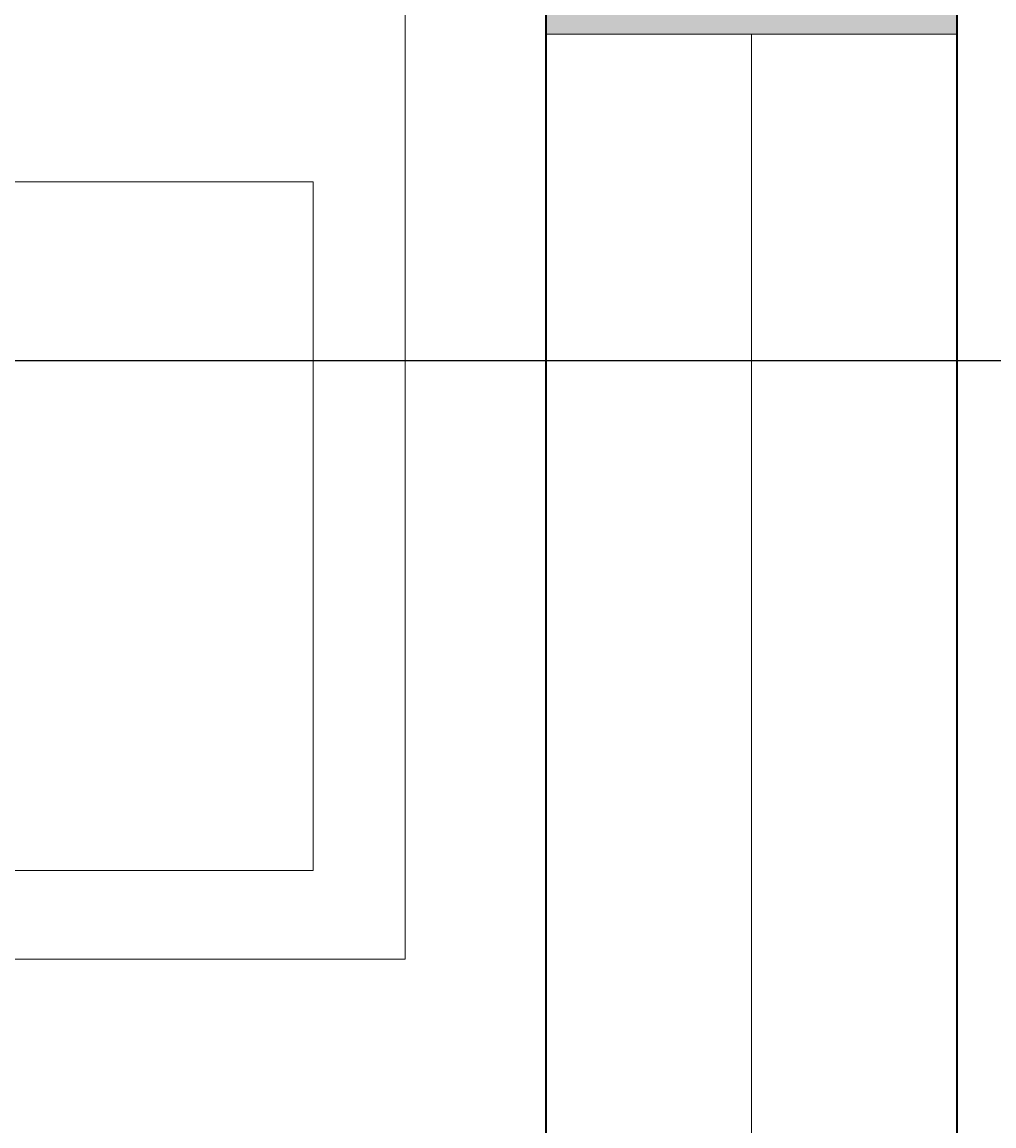
# Model space of a CAD drawing. Units: inches. Extents: x 1568 to 2529, y 2149 to 2897.
# Tile 11 of 16: x 1953 to 1974, y 2434 to 2459. Entities that reach past the tile are written whole.
import ezdxf

# ---------------------------------------------------------------- set-up
doc = ezdxf.new("R2010")
doc.units = ezdxf.units.IN
for name, color, linetype, lineweight in [('A-ANNO-DIMS', 2, 'Continuous', 18), ('A-FLOR-FIXT', 9, 'Continuous', 18), ('A-WALL-PATT', 172, 'Continuous', 13), ('wall', 7, 'Continuous', 35), ('window', 130, 'Continuous', 18)]:
    doc.layers.add(name, color=color, linetype=linetype, lineweight=lineweight)
doc.styles.get("Standard").update_dxf_attribs({"font": 'arial.ttf'})
doc.dimstyles.get("Standard").update_dxf_attribs({"dimtxt": 0.18, "dimasz": 0.18, "dimexe": 0.18, "dimexo": 0.0625, "dimgap": 0.09, "dimtad": 0, "dimtih": 1, "dimtoh": 1, "dimdec": 4, "dimzin": 0, "dimdsep": 46, "dimtxsty": 'Standard', "dimcen": 0.09, "dimadec": 0, "dimazin": 0, "dimtfac": 1, "dimtdec": 4, "dimtofl": 0, "dimtmove": 0, "dimatfit": 3, "dimfxl": 1, "dimtolj": 1, "dimtzin": 0, "dimarcsym": 0})

# ---------------------------------------------------------------- blocks, each defined once
blk = doc.blocks.new('*D28')
at = {"layer": 'A-ANNO-DIMS', "color": 0, "lineweight": -2, "transparency": 16777216}
for p, q in [((1973.643, 2801.532), (2009.61, 2801.532)), ((2009.43, 2801.352), (2009.43, 2501.714)), ((2009.43, 2201.712), (2009.43, 2501.35)), ((1973.613, 2201.532), (2009.61, 2201.532))]:
    blk.add_line(p, q, dxfattribs=at)
at = {"layer": 'A-ANNO-DIMS', "color": 0, "transparency": 16777216}
for points in [[(2009.4, 2801.352), (2009.46, 2801.352), (2009.43, 2801.532)], [(2009.4, 2201.712), (2009.46, 2201.712), (2009.43, 2201.532)]]:
    blk.add_solid(points, dxfattribs=at)
at = {"layer": 'Defpoints', "color": 0, "transparency": 16777216}
for p in [(1973.58, 2801.532), (2009.43, 2801.532), (1973.551, 2201.532)]:
    blk.add_point(p, dxfattribs=at)
at = {"layer": 'A-ANNO-DIMS', "color": 0, "transparency": 16777216, "insert": (2009.43, 2501.532), "char_height": 0.18, "attachment_point": 5}
blk.add_mtext('\\A1;600', dxfattribs=at)
blk = doc.blocks.new('*D32')
at = {"layer": 'A-ANNO-DIMS', "color": 0, "lineweight": -2, "transparency": 16777216}
for p, q in [((1964.551, 2792.469), (1964.551, 2165.502)), ((1904.551, 2753.401), (1904.551, 2165.502)), ((1904.731, 2165.682), (1934.332, 2165.682)), ((1964.371, 2165.682), (1934.77, 2165.682))]:
    blk.add_line(p, q, dxfattribs=at)
at = {"layer": 'A-ANNO-DIMS', "color": 0, "transparency": 16777216}
for points in [[(1904.731, 2165.712), (1904.731, 2165.652), (1904.551, 2165.682)], [(1964.371, 2165.712), (1964.371, 2165.652), (1964.551, 2165.682)]]:
    blk.add_solid(points, dxfattribs=at)
at = {"layer": 'Defpoints', "color": 0, "transparency": 16777216}
for p in [(1964.551, 2792.532), (1904.551, 2753.463), (1964.551, 2165.682)]:
    blk.add_point(p, dxfattribs=at)
at = {"layer": 'A-ANNO-DIMS', "color": 0, "transparency": 16777216, "insert": (1934.551, 2165.682), "char_height": 0.18, "attachment_point": 5}
blk.add_mtext('\\A1;60', dxfattribs=at)
blk = doc.blocks.new('*D35')
at = {"layer": 'A-ANNO-DIMS', "color": 0, "lineweight": -2, "transparency": 16777216}
for p, q in [((1759.113, 2451.227), (2009.61, 2451.227)), ((2009.43, 2451.047), (2009.43, 2431.409)), ((2009.43, 2411.407), (2009.43, 2431.045)), ((1759.113, 2411.227), (2009.61, 2411.227))]:
    blk.add_line(p, q, dxfattribs=at)
at = {"layer": 'A-ANNO-DIMS', "color": 0, "transparency": 16777216}
for points in [[(2009.4, 2451.047), (2009.46, 2451.047), (2009.43, 2451.227)], [(2009.4, 2411.407), (2009.46, 2411.407), (2009.43, 2411.227)]]:
    blk.add_solid(points, dxfattribs=at)
at = {"layer": 'Defpoints', "color": 0, "transparency": 16777216}
for p in [(1759.051, 2451.227), (2009.43, 2451.227), (1759.051, 2411.227)]:
    blk.add_point(p, dxfattribs=at)
at = {"layer": 'A-ANNO-DIMS', "color": 0, "transparency": 16777216, "insert": (2009.43, 2431.227), "char_height": 0.18, "attachment_point": 5}
blk.add_mtext('\\A1;40', dxfattribs=at)

msp = doc.modelspace()

# ---------------------------------------------------------------- hatches: boundary and pattern name
at = {"layer": 'A-WALL-PATT'}
h = msp.add_hatch(color=256, dxfattribs=at)
h.dxf.hatch_style = 1
h.paths.add_polyline_path([(1738.1593, 2801.532), (1634.4841, 2801.532), (1634.4841, 2792.532), (1738.1593, 2792.532)])
h.paths.add_polyline_path([(1812.4114, 2801.532), (1759.0925, 2801.532), (1759.0925, 2792.532), (1812.4114, 2792.532)])
h.paths.add_polyline_path([(1952.647, 2801.532), (1848.4114, 2801.532), (1848.4114, 2792.532), (1952.647, 2792.532)])
h.paths.add_polyline_path([(1973.5509, 2792.532), (1964.5509, 2792.532), (1964.5509, 2699.1671), (1973.5509, 2699.1671)])
h.paths.add_polyline_path([(1973.5509, 2663.1671), (1964.5509, 2663.1671), (1964.5509, 2630.5978), (1973.5509, 2630.5978)])
h.paths.add_polyline_path([(1973.5509, 2609.6646), (1964.5509, 2609.6646), (1964.5509, 2572.3679), (1973.5509, 2572.3679)])
h.paths.add_polyline_path([(1622.5509, 2753.3576), (1622.3864, 2753.3576), (1613.5509, 2753.3576), (1613.5509, 2705.9172), (1622.5509, 2705.9172)])
h.paths.add_polyline_path([(1622.5509, 2669.9172), (1613.5509, 2669.9172), (1613.5509, 2624.532), (1622.5509, 2624.532)])
h.paths.add_polyline_path([(1759.0509, 2757.9833), (1754.5509, 2757.9833), (1754.5509, 2744.532), (1622.5509, 2744.532), (1622.5509, 2740.032), (1754.5509, 2740.032), (1754.5509, 2730.8156), (1759.0509, 2730.8156), (1759.0509, 2740.032)])
h.paths.add_polyline_path([(1759.0509, 2690.8156), (1754.5509, 2690.8156), (1754.5509, 2624.532), (1759.0509, 2624.532)])
h.paths.add_polyline_path([(1738.1177, 2620.032), (1634.4841, 2620.032), (1634.4841, 2615.532), (1738.1177, 2615.532)])
h.paths.add_polyline_path([(1622.5509, 2615.532), (1613.5509, 2615.532), (1613.5509, 2564.2764), (1622.5509, 2564.2764)])
h.paths.add_polyline_path([(1759.0509, 2411.2271), (1754.5509, 2411.2271), (1754.5509, 2339.532), (1759.0509, 2339.532)])
h.paths.add_polyline_path([(1759.0509, 2464.032), (1734.3925, 2464.032), (1622.5509, 2464.032), (1622.5509, 2459.532), (1736.5509, 2459.532), (1754.5509, 2459.532), (1754.5509, 2451.2271), (1759.0509, 2451.2271)])
h.paths.add_polyline_path([(1844.5509, 2471.532), (1858.1805, 2471.532), (1858.1805, 2476.032), (1844.5509, 2476.032), (1844.5509, 2510.0763), (1840.0509, 2510.0763), (1840.0509, 2476.032), (1840.0509, 2339.532), (1844.5509, 2339.532)])
h.paths.add_polyline_path([(1844.5509, 2596.032), (1964.5509, 2596.032), (1964.5509, 2600.532), (1840.0509, 2600.532), (1840.0509, 2570.0763), (1844.5509, 2570.0763)])
h.paths.add_polyline_path([(1964.5509, 2476.032), (1894.1805, 2476.032), (1894.1805, 2471.532), (1964.5509, 2471.532)])
h.paths.add_polyline_path([(1622.5509, 2528.2764), (1613.5509, 2528.2764), (1613.5509, 2436.512), (1622.5509, 2436.512)])
h.paths.add_polyline_path([(1622.5509, 2400.512), (1613.5509, 2400.512), (1613.5509, 2339.532), (1622.5509, 2339.532)])
h.paths.add_polyline_path([(1738.9144, 2339.532), (1634.4841, 2339.532), (1634.4841, 2330.532), (1738.9144, 2330.532)])
h.paths.add_polyline_path([(1792.463, 2336.532, -0.0187698), (1792.5756, 2339.532), (1783.8928, 2339.532), (1783.8928, 2330.532), (1792.463, 2330.532)])
h.paths.add_polyline_path([(1952.6177, 2339.532), (1885.2912, 2339.532), (1885.2912, 2330.532), (1952.6177, 2330.532)])
h.paths.add_polyline_path([(1973.5509, 2422.371), (1964.5509, 2422.371), (1964.5509, 2395.032), (1964.5509, 2387.286), (1964.5509, 2339.532), (1973.5509, 2339.532)])
h.paths.add_polyline_path([(1973.5509, 2536.3679), (1964.5509, 2536.3679), (1964.5509, 2476.032), (1964.5509, 2458.371), (1973.5509, 2458.371)])

# ---------------------------------------------------------------- linework, layer by layer
at = {"layer": 'A-FLOR-FIXT'}
for points in [[(1941.7397, 2469.6671), (1961.4644, 2469.6671), (1961.4644, 2438.1142), (1941.7397, 2438.1142)], [(1943.5781, 2440.0573), (1959.4492, 2440.0573), (1959.4492, 2455.1398), (1943.5781, 2455.1398)]]:
    msp.add_lwpolyline(points, close=True, dxfattribs=at)
at = {"layer": 'wall'}
msp.add_lwpolyline([(1613.5509, 2201.532), (1973.5509, 2201.532), (1973.5509, 2801.532), (1613.5509, 2801.532)], close=True, dxfattribs=at)
msp.add_lwpolyline([(1964.5509, 2395.032), (1964.5509, 2792.532), (1622.5509, 2792.532), (1622.5509, 2624.532)], dxfattribs=at)
at = {"layer": 'window'}
for p, q in [((1964.5509, 2458.371), (1973.5509, 2458.371)), ((1969.0509, 2422.371), (1969.0509, 2458.371))]:
    msp.add_line(p, q, dxfattribs=at)

# ---------------------------------------------------------------- dimensions: what is measured, and where the dimension line sits
at = {"layer": 'A-ANNO-DIMS'}
for base, p1, p2, picture, middle in [((2009.4302, 2801.532), (1973.5509, 2201.532), (1973.5802, 2801.532), '*D28', (2009.4302, 2501.532)), ((2009.4302, 2451.2271), (1759.0509, 2411.2271), (1759.0509, 2451.2271), '*D35', (2009.4302, 2431.2271))]:
    dim = msp.add_linear_dim(base=base, p1=p1, p2=p2, angle=90, dimstyle='Standard', override={"dimdec": 0, "dimlfac": 1, "dimrnd": 0, "dimzin": 0, "dimdsep": 46, "dimlunit": 2}, dxfattribs=at)
    dim.commit()
    dim.dimension.update_dxf_attribs({"geometry": picture, "text_midpoint": middle})
dim = msp.add_linear_dim(base=(1964.5509, 2165.682), p1=(1904.5509, 2753.4635), p2=(1964.5509, 2792.532), dimstyle='Standard', override={"dimdec": 0, "dimlfac": 1, "dimrnd": 0, "dimzin": 0, "dimdsep": 46, "dimlunit": 2}, dxfattribs=at)
dim.commit()
dim.dimension.update_dxf_attribs({"geometry": '*D32', "text_midpoint": (1934.5509, 2165.682)})

doc.saveas('drawing.dxf')
